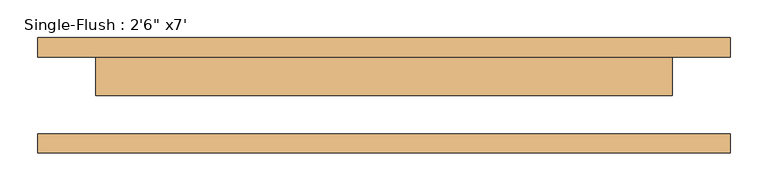
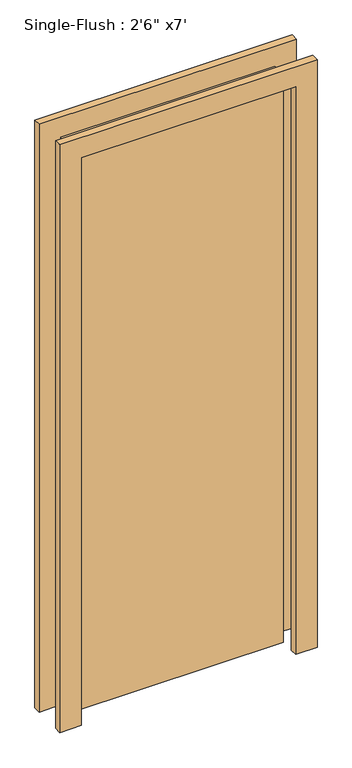
"""IFC4 building model written with IfcOpenShell, lengths in millimetres: door geometry."""

from ifc_helpers import new_model, si_unit, frame, origin, origin_with_axes, place, context, project, spatial, polyline, outline, extrude, source, transform, mapped, element, save


def door_270f2424(model_context):
    return source(origin(), model_context, "Body", "SweptSolid", [
        extrude(outline(polyline([(2209.8, -457.2), (0.0, -457.2), (0.0, -381.0), (2133.6, -381.0), (2133.6, 381.0), (0.0, 381.0), (0.0, 457.2), (2209.8, 457.2), (2209.8, -457.2)])), frame((0.0, 50.8, 0.0), z_axis=(0.0, 1.0, 0.0), x_axis=(0.0, 0.0, 1.0)), (0.0, 0.0, 1.0), 25.4),
        extrude(outline(polyline([(2209.8, 457.2), (2209.8, -457.2), (0.0, -457.2), (0.0, -381.0), (2133.6, -381.0), (2133.6, 381.0), (0.0, 381.0), (0.0, 457.2), (2209.8, 457.2)])), frame((0.0, -76.2, 0.0), z_axis=(0.0, 1.0, 0.0), x_axis=(0.0, 0.0, 1.0)), (0.0, 0.0, 1.0), 25.4),
        extrude(outline(polyline([(381.0, 0.0), (-381.0, 0.0), (-381.0, 50.8), (381.0, 50.8), (381.0, 0.0)])), origin_with_axes(), (0.0, 0.0, 1.0), 2133.6),
    ])


if __name__ == "__main__":
    model = new_model("IFC4")
    model_context = context("Model", 3, world=origin())
    ifc_project = project(units=[si_unit("LENGTHUNIT", "METRE", prefix="MILLI")], contexts=[model_context])
    site = spatial("IfcSite", under=ifc_project)
    building = spatial("IfcBuilding", under=site)
    placement = place(None, origin())
    door_shape = door_270f2424(model_context)
    element("IfcDoor", 1, ObjectType="Single-Flush : 2'6\" x7'", at=placement, inside=building, context=model_context, shape_type="MappedRepresentation", body=[
        mapped(door_shape, transform((0.0, 0.0, 0.0), x_axis=(1.0, 0.0, 0.0), y_axis=(0.0, 1.0, 0.0), z_axis=(0.0, 0.0, 1.0))),
    ])
    save(model, "model.ifc")

# Revit data of these elements
# Type "Single-Flush : 2'6\" x7'"
#   Type Mark = "15"
#   Construction Type Id = "MDOOR"
#   Assembly Code = "C1020"
#   Analytic Construction = "Metal"
#   Thickness = 0' - 2"
#   Heat Transfer Coefficient (U) = 0.651978 BTU/(h·ft²·°F)
#   Height = 7' - 0"
#   Trim Projection Ext = 0' - 1"
#   Trim Projection Int = 0' - 1"
#   Trim Width = 0' - 3"
#   Width = 2' - 6"
#   Define Thermal Properties by = 1
#   Door Material = Door - Panel
#   Frame Material = Door - Frame
#   Visual Light Transmittance = 0
#   Solar Heat Gain Coefficient = 0
#   Function = (empty or 0)
#   Wall Closure = (empty or 0)
# Element 1 (IfcDoor, "Single-Flush : 2'6\" x7'")
#   Materials on its faces: "Door - Frame", "Door - Panel"
# Materials
#   "Door - Panel": class "Wood", colour RGB 210 159 95, transparency 0, Cost = 0
#   "Door - Frame": colour RGB 118 70 51, transparency 0, Cost = 0
